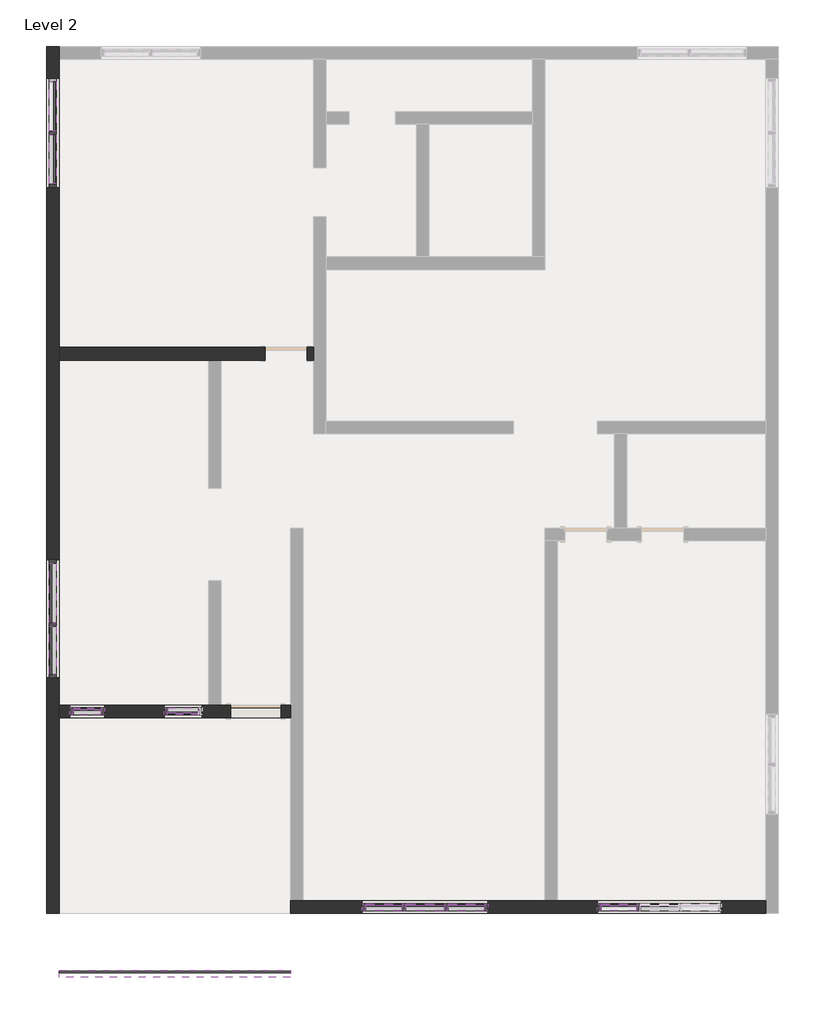
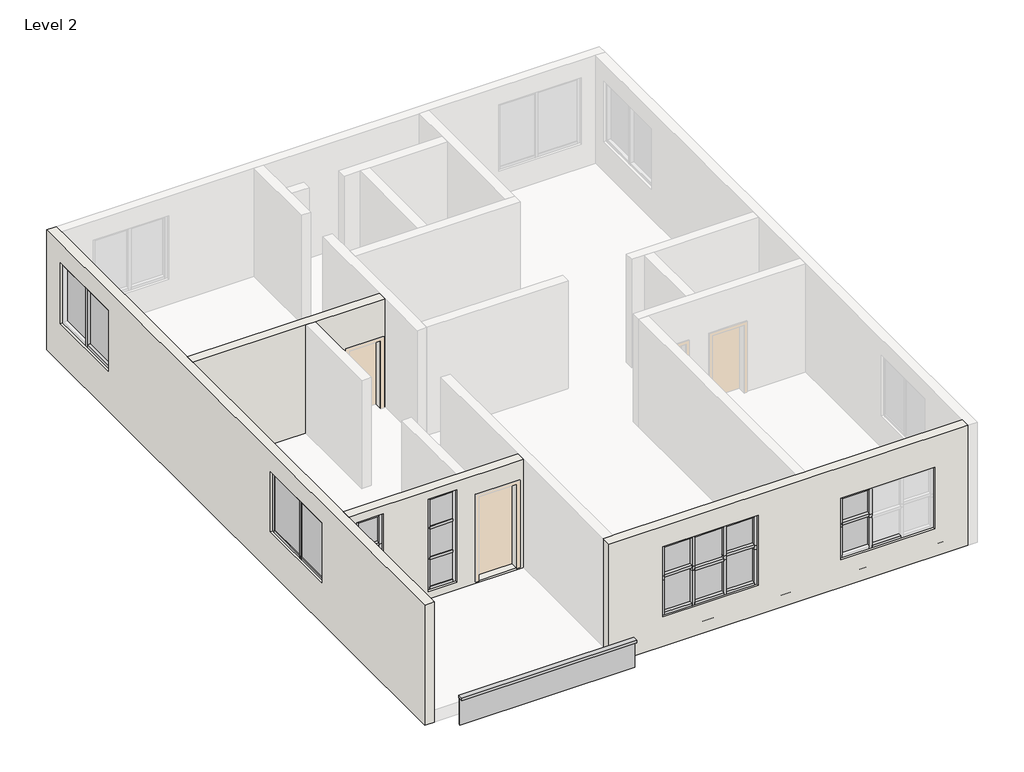
# One storey, part 1 of 2: 60 members, 19 plates, 4 walls.
"""IFC4 building model written with IfcOpenShell, lengths in millimetres."""

from ifc_helpers import new_model, si_unit, origin, place, context, project, spatial, faceted_brep, transform, mapped, element, save
from components import member_00d00b53, member_c7c5a8a0, member_b955a9e9, member_2ee2964b, member_c33c434a, member_3d7cb871, member_f1f71bde, member_024c663a, member_4d6ef9b1, member_a7b21902, member_e5016be8, member_72dfeae6, member_b41a733a, member_7fd687a9, member_90750a43, member_613aa8fe, member_6d419de8, member_bc554fa6, member_50cacee6, member_cfc5edb3, member_fb13da3b, member_24b317d4, member_58fda759, member_d6486fbc, member_c067c3a7, member_db897065, member_a044dc63, member_e51dd2bd, member_dfbe4da1, member_32677b83, member_f4ec938c, member_a37bde81, member_147bebee, system_panel_glazed_4c7522cd, system_panel_glazed_cbd410f7, system_panel_glazed_2af6040d, system_panel_glazed_3f6201ba, system_panel_glazed_11c7b7b5, system_panel_glazed_ea517728, system_panel_glazed_ffb4b76a, system_panel_glazed_52d1a9ac, system_panel_glazed_ee93d072, system_panel_glazed_cb6e72c2, system_panel_glazed_55fd798e, system_panel_glazed_d6f2290d, system_panel_glazed_2cf72723, system_panel_glazed_06e0175a

model = new_model("IFC4")

# Units and contexts
model_context = context("Model", 3, world=origin())
ifc_project = project(units=[si_unit("LENGTHUNIT", "METRE", prefix="MILLI")], contexts=[model_context])

# Site, building, storey
site = spatial("IfcSite", under=ifc_project)
building = spatial("IfcBuilding", under=site)
storey = spatial("IfcBuildingStorey", under=building, Name="Level 2", Elevation=3048.0)

# Members
placement = place(None, origin())
member_shape = member_00d00b53(model_context)
element("IfcMember", 1, ObjectType="Rectangular Mullion : 2.5\" x 5\" rectangular", at=placement, inside=storey, context=model_context, shape_type="MappedRepresentation", body=[
    mapped(member_shape, transform((-8069.267181, -14745.846149, 4532.9555732), x_axis=(1.0, 0.0, 0.0), y_axis=(0.0, -1.0, 0.0), z_axis=(0.0, 0.0, -1.0))),
])
member_2_shape = member_c7c5a8a0(model_context)
element("IfcMember", 2, ObjectType="Rectangular Mullion : 2.5\" x 5\" rectangular", at=placement, inside=storey, context=model_context, shape_type="MappedRepresentation", body=[
    mapped(member_2_shape, transform((-11593.6627168, -14745.846149, 4684.9213312), x_axis=(0.0, 0.0, 1.0), y_axis=(0.0, -1.0, 0.0), z_axis=(1.0, 0.0, 0.0))),
])
member_3_shape = member_b955a9e9(model_context)
element("IfcMember", 3, ObjectType="Rectangular Mullion : 2.5\" x 5\" rectangular", at=placement, inside=storey, context=model_context, shape_type="MappedRepresentation", body=[
    mapped(member_3_shape, transform((-11593.6627168, -14745.846149, 5574.6202549), x_axis=(0.0, 0.0, 1.0), y_axis=(0.0, -1.0, 0.0), z_axis=(1.0, 0.0, 0.0))),
])
element("IfcMember", 4, ObjectType="Rectangular Mullion : 2.5\" x 5\" rectangular", at=placement, inside=storey, context=model_context, shape_type="MappedRepresentation", body=[
    mapped(member_3_shape, transform((-12292.1627168, -14745.846149, 3795.2224075), x_axis=(0.0, 0.0, -1.0), y_axis=(0.0, -1.0, 0.0), z_axis=(-1.0, 0.0, 0.0))),
])
member_4_shape = member_2ee2964b(model_context)
element("IfcMember", 5, ObjectType="Rectangular Mullion : 2.5\" x 5\" rectangular", at=placement, inside=storey, context=model_context, shape_type="MappedRepresentation", body=[
    mapped(member_4_shape, transform((-10863.4127168, -14745.846149, 4786.5213312), x_axis=(0.0, 0.0, 1.0), y_axis=(0.0, -1.0, 0.0), z_axis=(1.0, 0.0, 0.0))),
])
element("IfcMember", 6, ObjectType="Rectangular Mullion : 2.5\" x 5\" rectangular", at=placement, inside=storey, context=model_context, shape_type="MappedRepresentation", body=[
    mapped(member_4_shape, transform((-12355.6627168, -14745.846149, 4786.5213312), x_axis=(0.0, 0.0, 1.0), y_axis=(0.0, -1.0, 0.0), z_axis=(1.0, 0.0, 0.0))),
])
member_5_shape = member_c33c434a(model_context)
element("IfcMember", 7, ObjectType="Rectangular Mullion : 2.5\" x 5\" rectangular", at=placement, inside=storey, context=model_context, shape_type="MappedRepresentation", body=[
    mapped(member_5_shape, transform((-12355.6627168, -14745.846149, 5574.6202549), x_axis=(0.0, 0.0, 1.0), y_axis=(0.0, -1.0, 0.0), z_axis=(1.0, 0.0, 0.0))),
])
element("IfcMember", 8, ObjectType="Rectangular Mullion : 2.5\" x 5\" rectangular", at=placement, inside=storey, context=model_context, shape_type="MappedRepresentation", body=[
    mapped(member_5_shape, transform((-10863.4127168, -14745.846149, 5574.6202549), x_axis=(0.0, 0.0, 1.0), y_axis=(0.0, -1.0, 0.0), z_axis=(1.0, 0.0, 0.0))),
])
element("IfcMember", 9, ObjectType="Rectangular Mullion : 2.5\" x 5\" rectangular", at=placement, inside=storey, context=model_context, shape_type="MappedRepresentation", body=[
    mapped(member_5_shape, transform((-11530.1627168, -14745.846149, 3795.2224075), x_axis=(0.0, 0.0, -1.0), y_axis=(0.0, -1.0, 0.0), z_axis=(-1.0, 0.0, 0.0))),
])
element("IfcMember", 10, ObjectType="Rectangular Mullion : 2.5\" x 5\" rectangular", at=placement, inside=storey, context=model_context, shape_type="MappedRepresentation", body=[
    mapped(member_5_shape, transform((-13022.4127168, -14745.846149, 3795.2224075), x_axis=(0.0, 0.0, -1.0), y_axis=(0.0, -1.0, 0.0), z_axis=(-1.0, 0.0, 0.0))),
])
member_6_shape = member_3d7cb871(model_context)
element("IfcMember", 11, ObjectType="Rectangular Mullion : 2.5\" x 5\" rectangular", at=placement, inside=storey, context=model_context, shape_type="MappedRepresentation", body=[
    mapped(member_6_shape, transform((-8818.7127168, -14745.846149, 4609.1555732), x_axis=(-1.0, 0.0, 0.0), y_axis=(0.0, -1.0, 0.0), z_axis=(0.0, 0.0, 1.0))),
])
member_7_shape = member_f1f71bde(model_context)
element("IfcMember", 12, ObjectType="Rectangular Mullion : 2.5\" x 5\" rectangular", at=placement, inside=storey, context=model_context, shape_type="MappedRepresentation", body=[
    mapped(member_7_shape, transform((-18686.1761094, -756.796149, 4059.4675701), x_axis=(0.0, 0.0, -1.0), y_axis=(-1.0, 0.0, 0.0), z_axis=(0.0, 1.0, 0.0))),
])
element("IfcMember", 13, ObjectType="Rectangular Mullion : 2.5\" x 5\" rectangular", at=placement, inside=storey, context=model_context, shape_type="MappedRepresentation", body=[
    mapped(member_7_shape, transform((-18686.1761094, -693.296149, 5599.1263641), x_axis=(0.0, 0.0, 1.0), y_axis=(-1.0, 0.0, 0.0), z_axis=(0.0, -1.0, 0.0))),
])
element("IfcMember", 14, ObjectType="Rectangular Mullion : 2.5\" x 5\" rectangular", at=placement, inside=storey, context=model_context, shape_type="MappedRepresentation", body=[
    mapped(member_7_shape, transform((-18686.1761094, -1652.146149, 5599.1263641), x_axis=(0.0, 0.0, 1.0), y_axis=(-1.0, 0.0, 0.0), z_axis=(0.0, -1.0, 0.0))),
])
member_8_shape = member_024c663a(model_context)
element("IfcMember", 15, ObjectType="Rectangular Mullion : 2.5\" x 5\" rectangular", at=placement, inside=storey, context=model_context, shape_type="MappedRepresentation", body=[
    mapped(member_8_shape, transform((-18686.1761094, -9659.496149, 5596.1060273), x_axis=(0.0, 0.0, 1.0), y_axis=(1.0, 0.0, 0.0), z_axis=(0.0, 1.0, 0.0))),
])
member_9_shape = member_4d6ef9b1(model_context)
element("IfcMember", 16, ObjectType="Rectangular Mullion : 2.5\" x 5\" rectangular", at=placement, inside=storey, context=model_context, shape_type="MappedRepresentation", body=[
    mapped(member_9_shape, transform((-18686.1761094, -8522.846149, 5596.1060273), x_axis=(0.0, 0.0, 1.0), y_axis=(1.0, 0.0, 0.0), z_axis=(0.0, 1.0, 0.0))),
])
member_10_shape = member_a7b21902(model_context)
element("IfcMember", 17, ObjectType="Rectangular Mullion : 2.5\" x 5\" rectangular", at=placement, inside=storey, context=model_context, shape_type="MappedRepresentation", body=[
    mapped(member_10_shape, transform((-18686.1761094, -9627.746149, 4073.0027042), x_axis=(0.0, 1.0, 0.0), y_axis=(1.0, 0.0, 0.0), z_axis=(0.0, 0.0, -1.0))),
])
element("IfcMember", 18, ObjectType="Rectangular Mullion : 2.5\" x 5\" rectangular", at=placement, inside=storey, context=model_context, shape_type="MappedRepresentation", body=[
    mapped(member_9_shape, transform((-18686.1761094, -9595.996149, 4073.0027042), x_axis=(0.0, 0.0, -1.0), y_axis=(1.0, 0.0, 0.0), z_axis=(0.0, -1.0, 0.0))),
])
element("IfcMember", 19, ObjectType="Rectangular Mullion : 2.5\" x 5\" rectangular", at=placement, inside=storey, context=model_context, shape_type="MappedRepresentation", body=[
    mapped(member_8_shape, transform((-18686.1761094, -10529.446149, 4073.0027042), x_axis=(0.0, 0.0, -1.0), y_axis=(1.0, 0.0, 0.0), z_axis=(0.0, -1.0, 0.0))),
])
member_11_shape = member_e5016be8(model_context)
element("IfcMember", 20, ObjectType="Rectangular Mullion : 2.5\" x 5\" rectangular", at=placement, inside=storey, context=model_context, shape_type="MappedRepresentation", body=[
    mapped(member_11_shape, transform((-18686.1761094, -10592.946149, 5596.1060273), x_axis=(0.0, -1.0, 0.0), y_axis=(1.0, 0.0, 0.0), z_axis=(0.0, 0.0, 1.0))),
])
element("IfcMember", 21, ObjectType="Rectangular Mullion : 2.5\" x 5\" rectangular", at=placement, inside=storey, context=model_context, shape_type="MappedRepresentation", body=[
    mapped(member_11_shape, transform((-18686.1761094, -8459.346149, 4073.0027042), x_axis=(0.0, 1.0, 0.0), y_axis=(1.0, 0.0, 0.0), z_axis=(0.0, 0.0, -1.0))),
])
member_12_shape = member_72dfeae6(model_context)
element("IfcMember", 22, ObjectType="Rectangular Mullion : 2.5\" x 5\" rectangular", at=placement, inside=storey, context=model_context, shape_type="MappedRepresentation", body=[
    mapped(member_12_shape, transform((-18686.1761094, -725.046149, 4059.4675701), x_axis=(0.0, -1.0, 0.0), y_axis=(-1.0, 0.0, 0.0), z_axis=(0.0, 0.0, -1.0))),
])
member_13_shape = member_b41a733a(model_context)
element("IfcMember", 23, ObjectType="Rectangular Mullion : 2.5\" x 5\" rectangular", at=placement, inside=storey, context=model_context, shape_type="MappedRepresentation", body=[
    mapped(member_13_shape, transform((-18686.1761094, -1715.646149, 4059.4675701), x_axis=(0.0, -1.0, 0.0), y_axis=(-1.0, 0.0, 0.0), z_axis=(0.0, 0.0, -1.0))),
])
member_14_shape = member_7fd687a9(model_context)
element("IfcMember", 24, ObjectType="Rectangular Mullion : 2.5\" x 5\" rectangular", at=placement, inside=storey, context=model_context, shape_type="MappedRepresentation", body=[
    mapped(member_14_shape, transform((-17809.8761094, -11202.546149, 5890.7358384), x_axis=(0.0, 0.0, 1.0), y_axis=(0.0, -1.0, 0.0), z_axis=(1.0, 0.0, 0.0))),
])
member_15_shape = member_90750a43(model_context)
element("IfcMember", 25, ObjectType="Rectangular Mullion : 2.5\" x 5\" rectangular", at=placement, inside=storey, context=model_context, shape_type="MappedRepresentation", body=[
    mapped(member_15_shape, transform((-17809.8761094, -11202.546149, 5114.1326107), x_axis=(0.0, 0.0, 1.0), y_axis=(0.0, -1.0, 0.0), z_axis=(1.0, 0.0, 0.0))),
])
element("IfcMember", 26, ObjectType="Rectangular Mullion : 2.5\" x 5\" rectangular", at=placement, inside=storey, context=model_context, shape_type="MappedRepresentation", body=[
    mapped(member_15_shape, transform((-17809.8761094, -11202.546149, 4337.5293829), x_axis=(0.0, 0.0, 1.0), y_axis=(0.0, -1.0, 0.0), z_axis=(1.0, 0.0, 0.0))),
])
member_16_shape = member_613aa8fe(model_context)
element("IfcMember", 27, ObjectType="Rectangular Mullion : 2.5\" x 5\" rectangular", at=placement, inside=storey, context=model_context, shape_type="MappedRepresentation", body=[
    mapped(member_16_shape, transform((-17746.3761094, -11202.546149, 5114.1326107), x_axis=(1.0, 0.0, 0.0), y_axis=(0.0, -1.0, 0.0), z_axis=(0.0, 0.0, -1.0))),
])
element("IfcMember", 28, ObjectType="Rectangular Mullion : 2.5\" x 5\" rectangular", at=placement, inside=storey, context=model_context, shape_type="MappedRepresentation", body=[
    mapped(member_16_shape, transform((-18381.3761094, -11202.546149, 5890.7358384), x_axis=(-1.0, 0.0, 0.0), y_axis=(0.0, -1.0, 0.0), z_axis=(0.0, 0.0, 1.0))),
])
element("IfcMember", 29, ObjectType="Rectangular Mullion : 2.5\" x 5\" rectangular", at=placement, inside=storey, context=model_context, shape_type="MappedRepresentation", body=[
    mapped(member_16_shape, transform((-17746.3761094, -11202.546149, 4337.5293829), x_axis=(1.0, 0.0, 0.0), y_axis=(0.0, -1.0, 0.0), z_axis=(0.0, 0.0, -1.0))),
])
element("IfcMember", 30, ObjectType="Rectangular Mullion : 2.5\" x 5\" rectangular", at=placement, inside=storey, context=model_context, shape_type="MappedRepresentation", body=[
    mapped(member_16_shape, transform((-18381.3761094, -11202.546149, 5114.1326107), x_axis=(-1.0, 0.0, 0.0), y_axis=(0.0, -1.0, 0.0), z_axis=(0.0, 0.0, 1.0))),
])
element("IfcMember", 31, ObjectType="Rectangular Mullion : 2.5\" x 5\" rectangular", at=placement, inside=storey, context=model_context, shape_type="MappedRepresentation", body=[
    mapped(member_14_shape, transform((-18317.8761094, -11202.546149, 3560.9261552), x_axis=(0.0, 0.0, -1.0), y_axis=(0.0, -1.0, 0.0), z_axis=(-1.0, 0.0, 0.0))),
])
element("IfcMember", 32, ObjectType="Rectangular Mullion : 2.5\" x 5\" rectangular", at=placement, inside=storey, context=model_context, shape_type="MappedRepresentation", body=[
    mapped(member_16_shape, transform((-17746.3761094, -11202.546149, 3560.9261552), x_axis=(1.0, 0.0, 0.0), y_axis=(0.0, -1.0, 0.0), z_axis=(0.0, 0.0, -1.0))),
])
element("IfcMember", 33, ObjectType="Rectangular Mullion : 2.5\" x 5\" rectangular", at=placement, inside=storey, context=model_context, shape_type="MappedRepresentation", body=[
    mapped(member_16_shape, transform((-18381.3761094, -11202.546149, 4337.5293829), x_axis=(-1.0, 0.0, 0.0), y_axis=(0.0, -1.0, 0.0), z_axis=(0.0, 0.0, 1.0))),
])
member_17_shape = member_6d419de8(model_context)
element("IfcMember", 34, ObjectType="Rectangular Mullion : 2.5\" x 5\" rectangular", at=placement, inside=storey, context=model_context, shape_type="MappedRepresentation", body=[
    mapped(member_17_shape, transform((-16666.8761094, -11202.546149, 5104.8752687), x_axis=(-1.0, 0.0, 0.0), y_axis=(0.0, 1.0, 0.0), z_axis=(0.0, 0.0, -1.0))),
])
member_18_shape = member_bc554fa6(model_context)
element("IfcMember", 35, ObjectType="Rectangular Mullion : 2.5\" x 5\" rectangular", at=placement, inside=storey, context=model_context, shape_type="MappedRepresentation", body=[
    mapped(member_18_shape, transform((-16603.3761094, -11202.546149, 5104.8752687), x_axis=(0.0, 0.0, 1.0), y_axis=(0.0, 1.0, 0.0), z_axis=(-1.0, 0.0, 0.0))),
])
element("IfcMember", 36, ObjectType="Rectangular Mullion : 2.5\" x 5\" rectangular", at=placement, inside=storey, context=model_context, shape_type="MappedRepresentation", body=[
    mapped(member_18_shape, transform((-16603.3761094, -11202.546149, 4324.942968), x_axis=(0.0, 0.0, 1.0), y_axis=(0.0, 1.0, 0.0), z_axis=(-1.0, 0.0, 0.0))),
])
member_19_shape = member_50cacee6(model_context)
element("IfcMember", 37, ObjectType="Rectangular Mullion : 2.5\" x 5\" rectangular", at=placement, inside=storey, context=model_context, shape_type="MappedRepresentation", body=[
    mapped(member_19_shape, transform((-16603.3761094, -11202.546149, 5884.8075695), x_axis=(0.0, 0.0, 1.0), y_axis=(0.0, 1.0, 0.0), z_axis=(-1.0, 0.0, 0.0))),
])
element("IfcMember", 38, ObjectType="Rectangular Mullion : 2.5\" x 5\" rectangular", at=placement, inside=storey, context=model_context, shape_type="MappedRepresentation", body=[
    mapped(member_17_shape, transform((-16666.8761094, -11202.546149, 4324.942968), x_axis=(-1.0, 0.0, 0.0), y_axis=(0.0, 1.0, 0.0), z_axis=(0.0, 0.0, -1.0))),
])
element("IfcMember", 39, ObjectType="Rectangular Mullion : 2.5\" x 5\" rectangular", at=placement, inside=storey, context=model_context, shape_type="MappedRepresentation", body=[
    mapped(member_19_shape, transform((-16044.5761094, -11202.546149, 3545.0106672), x_axis=(0.0, 0.0, -1.0), y_axis=(0.0, 1.0, 0.0), z_axis=(1.0, 0.0, 0.0))),
])
element("IfcMember", 40, ObjectType="Rectangular Mullion : 2.5\" x 5\" rectangular", at=placement, inside=storey, context=model_context, shape_type="MappedRepresentation", body=[
    mapped(member_17_shape, transform((-16666.8761094, -11202.546149, 3545.0106672), x_axis=(-1.0, 0.0, 0.0), y_axis=(0.0, 1.0, 0.0), z_axis=(0.0, 0.0, -1.0))),
])
member_20_shape = member_cfc5edb3(model_context)
element("IfcMember", 41, ObjectType="Rectangular Mullion : 2.5\" x 5\" rectangular", at=placement, inside=storey, context=model_context, shape_type="MappedRepresentation", body=[
    mapped(member_20_shape, transform((-12323.9127168, -14745.846149, 4684.9213312), x_axis=(1.0, 0.0, 0.0), y_axis=(0.0, -1.0, 0.0), z_axis=(0.0, 0.0, -1.0))),
])
element("IfcMember", 42, ObjectType="Rectangular Mullion : 2.5\" x 5\" rectangular", at=placement, inside=storey, context=model_context, shape_type="MappedRepresentation", body=[
    mapped(member_20_shape, transform((-11561.9127168, -14745.846149, 4684.9213312), x_axis=(1.0, 0.0, 0.0), y_axis=(0.0, -1.0, 0.0), z_axis=(0.0, 0.0, -1.0))),
])
member_21_shape = member_fb13da3b(model_context)
element("IfcMember", 43, ObjectType="Rectangular Mullion : 2.5\" x 5\" rectangular", at=placement, inside=storey, context=model_context, shape_type="MappedRepresentation", body=[
    mapped(member_21_shape, transform((-13085.9127168, -14745.846149, 4786.5213312), x_axis=(-1.0, 0.0, 0.0), y_axis=(0.0, -1.0, 0.0), z_axis=(0.0, 0.0, 1.0))),
])
member_22_shape = member_24b317d4(model_context)
element("IfcMember", 44, ObjectType="Rectangular Mullion : 2.5\" x 5\" rectangular", at=placement, inside=storey, context=model_context, shape_type="MappedRepresentation", body=[
    mapped(member_22_shape, transform((-12323.9127168, -14745.846149, 4786.5213312), x_axis=(1.0, 0.0, 0.0), y_axis=(0.0, -1.0, 0.0), z_axis=(0.0, 0.0, -1.0))),
])
element("IfcMember", 45, ObjectType="Rectangular Mullion : 2.5\" x 5\" rectangular", at=placement, inside=storey, context=model_context, shape_type="MappedRepresentation", body=[
    mapped(member_22_shape, transform((-11561.9127168, -14745.846149, 4786.5213312), x_axis=(1.0, 0.0, 0.0), y_axis=(0.0, -1.0, 0.0), z_axis=(0.0, 0.0, -1.0))),
])
member_23_shape = member_58fda759(model_context)
element("IfcMember", 46, ObjectType="Rectangular Mullion : 2.5\" x 5\" rectangular", at=placement, inside=storey, context=model_context, shape_type="MappedRepresentation", body=[
    mapped(member_23_shape, transform((-13085.9127168, -14745.846149, 5574.6202549), x_axis=(-1.0, 0.0, 0.0), y_axis=(0.0, -1.0, 0.0), z_axis=(0.0, 0.0, 1.0))),
])
element("IfcMember", 47, ObjectType="Rectangular Mullion : 2.5\" x 5\" rectangular", at=placement, inside=storey, context=model_context, shape_type="MappedRepresentation", body=[
    mapped(member_23_shape, transform((-10799.9127168, -14745.846149, 4786.5213312), x_axis=(1.0, 0.0, 0.0), y_axis=(0.0, -1.0, 0.0), z_axis=(0.0, 0.0, -1.0))),
])
element("IfcMember", 48, ObjectType="Rectangular Mullion : 2.5\" x 5\" rectangular", at=placement, inside=storey, context=model_context, shape_type="MappedRepresentation", body=[
    mapped(member_21_shape, transform((-10799.9127168, -14745.846149, 4684.9213312), x_axis=(1.0, 0.0, 0.0), y_axis=(0.0, -1.0, 0.0), z_axis=(0.0, 0.0, -1.0))),
])
member_24_shape = member_d6486fbc(model_context)
element("IfcMember", 49, ObjectType="Rectangular Mullion : 2.5\" x 5\" rectangular", at=placement, inside=storey, context=model_context, shape_type="MappedRepresentation", body=[
    mapped(member_24_shape, transform((-12323.9127168, -14745.846149, 3795.2224075), x_axis=(1.0, 0.0, 0.0), y_axis=(0.0, -1.0, 0.0), z_axis=(0.0, 0.0, -1.0))),
])
element("IfcMember", 50, ObjectType="Rectangular Mullion : 2.5\" x 5\" rectangular", at=placement, inside=storey, context=model_context, shape_type="MappedRepresentation", body=[
    mapped(member_24_shape, transform((-11561.9127168, -14745.846149, 3795.2224075), x_axis=(1.0, 0.0, 0.0), y_axis=(0.0, -1.0, 0.0), z_axis=(0.0, 0.0, -1.0))),
])
member_25_shape = member_c067c3a7(model_context)
element("IfcMember", 51, ObjectType="Rectangular Mullion : 2.5\" x 5\" rectangular", at=placement, inside=storey, context=model_context, shape_type="MappedRepresentation", body=[
    mapped(member_25_shape, transform((-13085.9127168, -14745.846149, 4684.9213312), x_axis=(-1.0, 0.0, 0.0), y_axis=(0.0, -1.0, 0.0), z_axis=(0.0, 0.0, 1.0))),
])
element("IfcMember", 52, ObjectType="Rectangular Mullion : 2.5\" x 5\" rectangular", at=placement, inside=storey, context=model_context, shape_type="MappedRepresentation", body=[
    mapped(member_25_shape, transform((-10799.9127168, -14745.846149, 3795.2224075), x_axis=(1.0, 0.0, 0.0), y_axis=(0.0, -1.0, 0.0), z_axis=(0.0, 0.0, -1.0))),
])
member_26_shape = member_db897065(model_context)
element("IfcMember", 53, ObjectType="Rectangular Mullion : 2.5\" x 5\" rectangular", at=placement, inside=storey, context=model_context, shape_type="MappedRepresentation", body=[
    mapped(member_26_shape, transform((-8069.267181, -14745.846149, 4609.1555732), x_axis=(1.0, 0.0, 0.0), y_axis=(0.0, -1.0, 0.0), z_axis=(0.0, 0.0, -1.0))),
])
member_27_shape = member_a044dc63(model_context)
element("IfcMember", 54, ObjectType="Rectangular Mullion : 2.5\" x 5\" rectangular", at=placement, inside=storey, context=model_context, shape_type="MappedRepresentation", body=[
    mapped(member_27_shape, transform((-8101.017181, -14745.846149, 5311.3816242), x_axis=(0.0, 0.0, 1.0), y_axis=(0.0, -1.0, 0.0), z_axis=(1.0, 0.0, 0.0))),
])
member_28_shape = member_e51dd2bd(model_context)
element("IfcMember", 55, ObjectType="Rectangular Mullion : 2.5\" x 5\" rectangular", at=placement, inside=storey, context=model_context, shape_type="MappedRepresentation", body=[
    mapped(member_28_shape, transform((-8101.017181, -14745.846149, 4609.1555732), x_axis=(0.0, 0.0, 1.0), y_axis=(0.0, -1.0, 0.0), z_axis=(1.0, 0.0, 0.0))),
])
member_29_shape = member_dfbe4da1(model_context)
element("IfcMember", 56, ObjectType="Rectangular Mullion : 2.5\" x 5\" rectangular", at=placement, inside=storey, context=model_context, shape_type="MappedRepresentation", body=[
    mapped(member_29_shape, transform((-8818.7127168, -14745.846149, 5311.3816242), x_axis=(-1.0, 0.0, 0.0), y_axis=(0.0, -1.0, 0.0), z_axis=(0.0, 0.0, 1.0))),
])
member_30_shape = member_32677b83(model_context)
element("IfcMember", 57, ObjectType="Rectangular Mullion : 2.5\" x 5\" rectangular", at=placement, inside=storey, context=model_context, shape_type="MappedRepresentation", body=[
    mapped(member_30_shape, transform((-8069.267181, -14745.846149, 3754.5295223), x_axis=(1.0, 0.0, 0.0), y_axis=(0.0, -1.0, 0.0), z_axis=(0.0, 0.0, -1.0))),
])
member_31_shape = member_f4ec938c(model_context)
element("IfcMember", 58, ObjectType="Rectangular Mullion : 2.5\" x 5\" rectangular", at=placement, inside=storey, context=model_context, shape_type="MappedRepresentation", body=[
    mapped(member_31_shape, transform((-8037.517181, -14745.846149, 3754.5295223), x_axis=(0.0, 0.0, -1.0), y_axis=(0.0, -1.0, 0.0), z_axis=(-1.0, 0.0, 0.0))),
])
member_32_shape = member_a37bde81(model_context)
element("IfcMember", 59, ObjectType="Rectangular Mullion : 2.5\" x 5\" rectangular", at=placement, inside=storey, context=model_context, shape_type="MappedRepresentation", body=[
    mapped(member_32_shape, transform((-8818.7127168, -14745.846149, 4532.9555732), x_axis=(-1.0, 0.0, 0.0), y_axis=(0.0, -1.0, 0.0), z_axis=(0.0, 0.0, 1.0))),
])
member_33_shape = member_147bebee(model_context)
element("IfcMember", 60, ObjectType="Rectangular Mullion : 2.5\" x 5\" rectangular", at=placement, inside=storey, context=model_context, shape_type="MappedRepresentation", body=[
    mapped(member_33_shape, transform((-14380.8761094, -15957.1913837, 4356.692968), x_axis=(0.0, 0.0, 1.0), y_axis=(0.0, -1.0, 0.0), z_axis=(1.0, 0.0, 0.0))),
])

# Plates
system_panel_glazed_shape = system_panel_glazed_4c7522cd(model_context)
element("IfcPlate", 61, ObjectType="System Panel : Glazed", at=placement, inside=storey, context=model_context, shape_type="MappedRepresentation", body=[
    mapped(system_panel_glazed_shape, transform((-18686.1761094, -10094.471149, 4136.5027042), x_axis=(0.0, 1.0, 0.0), y_axis=(-1.0, 0.0, 0.0), z_axis=(0.0, 0.0, 1.0))),
])
system_panel_glazed_2_shape = system_panel_glazed_cbd410f7(model_context)
element("IfcPlate", 62, ObjectType="System Panel : Glazed", at=placement, inside=storey, context=model_context, shape_type="MappedRepresentation", body=[
    mapped(system_panel_glazed_2_shape, transform((-18686.1761094, -9059.421149, 4136.5027042), x_axis=(0.0, 1.0, 0.0), y_axis=(-1.0, 0.0, 0.0), z_axis=(0.0, 0.0, 1.0))),
])
system_panel_glazed_3_shape = system_panel_glazed_2af6040d(model_context)
element("IfcPlate", 63, ObjectType="System Panel : Glazed", at=placement, inside=storey, context=model_context, shape_type="MappedRepresentation", body=[
    mapped(system_panel_glazed_3_shape, transform((-18686.1761094, -245.621149, 4122.9675701), x_axis=(0.0, -1.0, 0.0), y_axis=(1.0, 0.0, 0.0), z_axis=(0.0, 0.0, 1.0))),
])
element("IfcPlate", 64, ObjectType="System Panel : Glazed", at=placement, inside=storey, context=model_context, shape_type="MappedRepresentation", body=[
    mapped(system_panel_glazed_3_shape, transform((-18686.1761094, -1204.471149, 4122.9675701), x_axis=(0.0, -1.0, 0.0), y_axis=(1.0, 0.0, 0.0), z_axis=(0.0, 0.0, 1.0))),
])
system_panel_glazed_4_shape = system_panel_glazed_3f6201ba(model_context)
element("IfcPlate", 65, ObjectType="System Panel : Glazed", at=placement, inside=storey, context=model_context, shape_type="MappedRepresentation", body=[
    mapped(system_panel_glazed_4_shape, transform((-18063.8761094, -11202.546149, 3624.4261552), x_axis=(1.0, 0.0, 0.0), y_axis=(0.0, 1.0, 0.0), z_axis=(0.0, 0.0, 1.0))),
])
element("IfcPlate", 66, ObjectType="System Panel : Glazed", at=placement, inside=storey, context=model_context, shape_type="MappedRepresentation", body=[
    mapped(system_panel_glazed_4_shape, transform((-18063.8761094, -11202.546149, 5145.8826107), x_axis=(1.0, 0.0, 0.0), y_axis=(0.0, 1.0, 0.0), z_axis=(0.0, 0.0, 1.0))),
])
system_panel_glazed_5_shape = system_panel_glazed_11c7b7b5(model_context)
element("IfcPlate", 67, ObjectType="System Panel : Glazed", at=placement, inside=storey, context=model_context, shape_type="MappedRepresentation", body=[
    mapped(system_panel_glazed_5_shape, transform((-18063.8761094, -11202.546149, 4369.2793829), x_axis=(1.0, 0.0, 0.0), y_axis=(0.0, 1.0, 0.0), z_axis=(0.0, 0.0, 1.0))),
])
system_panel_glazed_6_shape = system_panel_glazed_ea517728(model_context)
element("IfcPlate", 68, ObjectType="System Panel : Glazed", at=placement, inside=storey, context=model_context, shape_type="MappedRepresentation", body=[
    mapped(system_panel_glazed_6_shape, transform((-16323.9761094, -11202.546149, 3608.5106672), x_axis=(-1.0, 0.0, 0.0), y_axis=(0.0, -1.0, 0.0), z_axis=(0.0, 0.0, 1.0))),
])
element("IfcPlate", 69, ObjectType="System Panel : Glazed", at=placement, inside=storey, context=model_context, shape_type="MappedRepresentation", body=[
    mapped(system_panel_glazed_6_shape, transform((-16323.9761094, -11202.546149, 5136.6252687), x_axis=(-1.0, 0.0, 0.0), y_axis=(0.0, -1.0, 0.0), z_axis=(0.0, 0.0, 1.0))),
])
system_panel_glazed_7_shape = system_panel_glazed_ffb4b76a(model_context)
element("IfcPlate", 70, ObjectType="System Panel : Glazed", at=placement, inside=storey, context=model_context, shape_type="MappedRepresentation", body=[
    mapped(system_panel_glazed_7_shape, transform((-16323.9761094, -11202.546149, 4356.692968), x_axis=(-1.0, 0.0, 0.0), y_axis=(0.0, -1.0, 0.0), z_axis=(0.0, 0.0, 1.0))),
])
system_panel_glazed_8_shape = system_panel_glazed_52d1a9ac(model_context)
element("IfcPlate", 71, ObjectType="System Panel : Glazed", at=placement, inside=storey, context=model_context, shape_type="MappedRepresentation", body=[
    mapped(system_panel_glazed_8_shape, transform((-12689.0377168, -14745.846149, 4818.2713312), x_axis=(1.0, 0.0, 0.0), y_axis=(0.0, 1.0, 0.0), z_axis=(0.0, 0.0, 1.0))),
])
element("IfcPlate", 72, ObjectType="System Panel : Glazed", at=placement, inside=storey, context=model_context, shape_type="MappedRepresentation", body=[
    mapped(system_panel_glazed_8_shape, transform((-11196.7877168, -14745.846149, 4818.2713312), x_axis=(1.0, 0.0, 0.0), y_axis=(0.0, 1.0, 0.0), z_axis=(0.0, 0.0, 1.0))),
])
system_panel_glazed_9_shape = system_panel_glazed_ee93d072(model_context)
element("IfcPlate", 73, ObjectType="System Panel : Glazed", at=placement, inside=storey, context=model_context, shape_type="MappedRepresentation", body=[
    mapped(system_panel_glazed_9_shape, transform((-11942.9127168, -14745.846149, 4716.6713312), x_axis=(1.0, 0.0, 0.0), y_axis=(0.0, 1.0, 0.0), z_axis=(0.0, 0.0, 1.0))),
])
system_panel_glazed_10_shape = system_panel_glazed_cb6e72c2(model_context)
element("IfcPlate", 74, ObjectType="System Panel : Glazed", at=placement, inside=storey, context=model_context, shape_type="MappedRepresentation", body=[
    mapped(system_panel_glazed_10_shape, transform((-12689.0377168, -14745.846149, 3858.7224075), x_axis=(1.0, 0.0, 0.0), y_axis=(0.0, 1.0, 0.0), z_axis=(0.0, 0.0, 1.0))),
])
element("IfcPlate", 75, ObjectType="System Panel : Glazed", at=placement, inside=storey, context=model_context, shape_type="MappedRepresentation", body=[
    mapped(system_panel_glazed_10_shape, transform((-11196.7877168, -14745.846149, 3858.7224075), x_axis=(1.0, 0.0, 0.0), y_axis=(0.0, 1.0, 0.0), z_axis=(0.0, 0.0, 1.0))),
])
system_panel_glazed_11_shape = system_panel_glazed_55fd798e(model_context)
element("IfcPlate", 76, ObjectType="System Panel : Glazed", at=placement, inside=storey, context=model_context, shape_type="MappedRepresentation", body=[
    mapped(system_panel_glazed_11_shape, transform((-11942.9127168, -14745.846149, 3858.7224075), x_axis=(1.0, 0.0, 0.0), y_axis=(0.0, 1.0, 0.0), z_axis=(0.0, 0.0, 1.0))),
])
system_panel_glazed_12_shape = system_panel_glazed_d6f2290d(model_context)
element("IfcPlate", 77, ObjectType="System Panel : Glazed", at=placement, inside=storey, context=model_context, shape_type="MappedRepresentation", body=[
    mapped(system_panel_glazed_12_shape, transform((-8428.1149489, -14745.846149, 4640.9055732), x_axis=(1.0, 0.0, 0.0), y_axis=(0.0, 1.0, 0.0), z_axis=(0.0, 0.0, 1.0))),
])
system_panel_glazed_13_shape = system_panel_glazed_2cf72723(model_context)
element("IfcPlate", 78, ObjectType="System Panel : Glazed", at=placement, inside=storey, context=model_context, shape_type="MappedRepresentation", body=[
    mapped(system_panel_glazed_13_shape, transform((-8428.1149489, -14745.846149, 3818.0295223), x_axis=(1.0, 0.0, 0.0), y_axis=(0.0, 1.0, 0.0), z_axis=(0.0, 0.0, 1.0))),
])
system_panel_glazed_14_shape = system_panel_glazed_06e0175a(model_context)
element("IfcPlate", 79, ObjectType="System Panel : Glazed", at=placement, inside=storey, context=model_context, shape_type="MappedRepresentation", body=[
    mapped(system_panel_glazed_14_shape, transform((-16476.3761094, -15957.1913837, 3630.9088336), x_axis=(1.0, 0.0, 0.0), y_axis=(0.0, 1.0, 0.0), z_axis=(0.0, 0.0, 1.0))),
])

# Walls
element("IfcWall", 80, ObjectType="9\"", at=placement, inside=storey, context=model_context, shape_type="Brep", body=[
    faceted_brep([(-18571.8761094, -14860.146149, 3048.0), (-18571.8761094, -11316.846149, 3048.0), (-18571.8761094, -11088.246149, 3048.0), (-18571.8761094, -4839.846149, 3048.0), (-18571.8761094, -4611.246149, 3048.0), (-18571.8761094, 608.453851, 3048.0), (-18571.8761094, 837.053851, 3048.0), (-18571.8761094, 837.053851, 6096.0), (-18571.8761094, 608.453851, 6096.0), (-18571.8761094, -4611.246149, 6096.0), (-18571.8761094, -4839.846149, 6096.0), (-18571.8761094, -11088.246149, 6096.0), (-18571.8761094, -11316.846149, 6096.0), (-18571.8761094, -14860.146149, 6096.0), (-18571.8761094, 265.553851, 5599.1263641), (-18571.8761094, 265.553851, 4059.4675701), (-18571.8761094, -1715.646149, 4059.4675701), (-18571.8761094, -1715.646149, 5599.1263641), (-18571.8761094, -10592.946149, 4073.0027042), (-18571.8761094, -10592.946149, 5596.1060273), (-18571.8761094, -8459.346149, 5596.1060273), (-18571.8761094, -8459.346149, 4073.0027042), (-18800.4761094, 837.053851, 3048.0), (-18800.4761094, -14860.146149, 3048.0), (-18800.4761094, -14860.146149, 6096.0), (-18800.4761094, 837.053851, 6096.0), (-18800.4761094, 265.553851, 4059.4675701), (-18800.4761094, 265.553851, 5599.1263641), (-18800.4761094, -1715.646149, 5599.1263641), (-18800.4761094, -1715.646149, 4059.4675701), (-18800.4761094, -10592.946149, 5596.1060273), (-18800.4761094, -10592.946149, 4073.0027042), (-18800.4761094, -8459.346149, 4073.0027042), (-18800.4761094, -8459.346149, 5596.1060273)], [[[0, 1, 2, 3, 4, 5, 6, 7, 8, 9, 10, 11, 12, 13], [14, 15, 16, 17], [18, 19, 20, 21]], [[22, 23, 24, 25], [26, 27, 28, 29], [30, 31, 32, 33]], [[6, 5, 4, 3, 2, 1, 0, 23, 22]], [[13, 12, 11, 10, 9, 8, 7, 25, 24]], [[0, 13, 24, 23]], [[7, 6, 22, 25]], [[26, 15, 14, 27]], [[27, 14, 17, 28]], [[28, 17, 16, 29]], [[15, 26, 29, 16]], [[30, 19, 18, 31]], [[19, 30, 33, 20]], [[20, 33, 32, 21]], [[31, 18, 21, 32]]]),
])
element("IfcWall", 81, ObjectType="9\"", at=placement, inside=storey, context=model_context, shape_type="Brep", body=[
    faceted_brep([(-5770.2761094, -14631.546149, 3048.0), (-9542.1761094, -14631.546149, 3048.0), (-9770.7761094, -14631.546149, 3048.0), (-14152.2761094, -14631.546149, 3048.0), (-14380.8761094, -14631.546149, 3048.0), (-14380.8761094, -14631.546149, 6096.0), (-14152.2761094, -14631.546149, 6096.0), (-9770.7761094, -14631.546149, 6096.0), (-9542.1761094, -14631.546149, 6096.0), (-5770.2761094, -14631.546149, 6096.0), (-13085.9127168, -14631.546149, 5574.6202549), (-13085.9127168, -14631.546149, 3795.2224075), (-10799.9127168, -14631.546149, 3795.2224075), (-10799.9127168, -14631.546149, 5574.6202549), (-8818.7127168, -14631.546149, 5311.3816242), (-8818.7127168, -14631.546149, 3754.5295223), (-6570.3761094, -14631.546149, 3754.5295223), (-6570.3761094, -14631.546149, 5311.3816242), (-14380.8761094, -14860.146149, 3048.0), (-5770.2761094, -14860.146149, 3048.0), (-5770.2761094, -14860.146149, 6096.0), (-14380.8761094, -14860.146149, 6096.0), (-13085.9127168, -14860.146149, 3795.2224075), (-13085.9127168, -14860.146149, 5574.6202549), (-10799.9127168, -14860.146149, 5574.6202549), (-10799.9127168, -14860.146149, 3795.2224075), (-8818.7127168, -14860.146149, 3754.5295223), (-8818.7127168, -14860.146149, 5311.3816242), (-6570.3761094, -14860.146149, 5311.3816242), (-6570.3761094, -14860.146149, 3754.5295223)], [[[0, 1, 2, 3, 4, 5, 6, 7, 8, 9], [10, 11, 12, 13], [14, 15, 16, 17]], [[18, 19, 20, 21], [22, 23, 24, 25], [26, 27, 28, 29]], [[4, 3, 2, 1, 0, 19, 18]], [[9, 8, 7, 6, 5, 21, 20]], [[0, 9, 20, 19]], [[5, 4, 18, 21]], [[10, 23, 22, 11]], [[23, 10, 13, 24]], [[24, 13, 12, 25]], [[11, 22, 25, 12]], [[26, 15, 14, 27]], [[27, 14, 17, 28]], [[28, 17, 16, 29]], [[15, 26, 29, 16]]]),
])
element("IfcWall", 82, ObjectType="9\"", at=placement, inside=storey, context=model_context, shape_type="Brep", body=[
    faceted_brep([(-14380.8761094, -11088.246149, 3048.0), (-15638.1761094, -11088.246149, 3048.0), (-15866.7761094, -11088.246149, 3048.0), (-18571.8761094, -11088.246149, 3048.0), (-18571.8761094, -11088.246149, 6096.0), (-15866.7761094, -11088.246149, 6096.0), (-15638.1761094, -11088.246149, 6096.0), (-14380.8761094, -11088.246149, 6096.0), (-15466.7261094, -11088.246149, 3403.6), (-14552.3261094, -11088.246149, 3403.6), (-14552.3261094, -11088.246149, 5537.2), (-15466.7261094, -11088.246149, 5537.2), (-15981.0761094, -11088.246149, 3545.0106672), (-15981.0761094, -11088.246149, 5884.8075695), (-16666.8761094, -11088.246149, 5884.8075695), (-16666.8761094, -11088.246149, 3545.0106672), (-18381.3761094, -11088.246149, 5890.7358384), (-18381.3761094, -11088.246149, 3560.9261552), (-17746.3761094, -11088.246149, 3560.9261552), (-17746.3761094, -11088.246149, 5890.7358384), (-18571.8761094, -11316.846149, 3048.0), (-14380.8761094, -11316.846149, 3048.0), (-14380.8761094, -11316.846149, 6096.0), (-18571.8761094, -11316.846149, 6096.0), (-14552.3261094, -11316.846149, 3403.6), (-15466.7261094, -11316.846149, 3403.6), (-15466.7261094, -11316.846149, 5537.2), (-14552.3261094, -11316.846149, 5537.2), (-15981.0761094, -11316.846149, 5884.8075695), (-15981.0761094, -11316.846149, 3545.0106672), (-16666.8761094, -11316.846149, 3545.0106672), (-16666.8761094, -11316.846149, 5884.8075695), (-18381.3761094, -11316.846149, 3560.9261552), (-18381.3761094, -11316.846149, 5890.7358384), (-17746.3761094, -11316.846149, 5890.7358384), (-17746.3761094, -11316.846149, 3560.9261552)], [[[0, 1, 2, 3, 4, 5, 6, 7], [8, 9, 10, 11], [12, 13, 14, 15], [16, 17, 18, 19]], [[20, 21, 22, 23], [24, 25, 26, 27], [28, 29, 30, 31], [32, 33, 34, 35]], [[3, 2, 1, 0, 21, 20]], [[7, 6, 5, 4, 23, 22]], [[0, 7, 22, 21]], [[4, 3, 20, 23]], [[9, 8, 25, 24]], [[10, 9, 24, 27]], [[11, 10, 27, 26]], [[8, 11, 26, 25]], [[12, 29, 28, 13]], [[13, 28, 31, 14]], [[14, 31, 30, 15]], [[29, 12, 15, 30]], [[32, 17, 16, 33]], [[33, 16, 19, 34]], [[18, 35, 34, 19]], [[17, 32, 35, 18]]]),
])
element("IfcWall", 83, ObjectType="9\"", at=placement, inside=storey, context=model_context, shape_type="Brep", body=[
    faceted_brep([(-14076.5127168, -4839.846149, 5080.0), (-14076.5127168, -4839.846149, 3048.0), (-13962.2127168, -4839.846149, 3048.0), (-13962.2127168, -4839.846149, 6096.0), (-15638.1761094, -4839.846149, 6096.0), (-15866.7761094, -4839.846149, 6096.0), (-18571.8761094, -4839.846149, 6096.0), (-18571.8761094, -4839.846149, 3048.0), (-15866.7761094, -4839.846149, 3048.0), (-15638.1761094, -4839.846149, 3048.0), (-14838.5127168, -4839.846149, 3048.0), (-14838.5127168, -4839.846149, 5080.0), (-13962.2127168, -4611.246149, 3048.0), (-14076.5127168, -4611.246149, 3048.0), (-14076.5127168, -4611.246149, 5080.0), (-14838.5127168, -4611.246149, 5080.0), (-14838.5127168, -4611.246149, 3048.0), (-18571.8761094, -4611.246149, 3048.0), (-18571.8761094, -4611.246149, 6096.0), (-13962.2127168, -4611.246149, 6096.0)], [[[0, 1, 2, 3, 4, 5, 6, 7, 8, 9, 10, 11]], [[12, 13, 14, 15, 16, 17, 18, 19]], [[2, 1, 13, 12]], [[10, 9, 8, 7, 17, 16]], [[6, 5, 4, 3, 19, 18]], [[7, 6, 18, 17]], [[3, 2, 12, 19]], [[14, 13, 1, 0]], [[15, 14, 0, 11]], [[16, 15, 11, 10]]]),
])

save(model, "model.ifc")

# Revit data of these elements
# Type "Rectangular Mullion : 2.5\" x 5\" rectangular"
#   built-in parameter 1007304 = 0.416667 (stored number, unit not read)
#   built-in parameter 1007301 = 0.104167 (stored number, unit not read)
#   built-in parameter 1007300 = 0.104167 (stored number, unit not read)
# Type "System Panel : Glazed"
#   Construction Type Id = "GSP4R"
#   Analytic Construction = "1/8 in Pilkington single glazing"
#   Visual Light Transmittance = 0.9
#   Solar Heat Gain Coefficient = 0.86
#   Heat Transfer Coefficient (U) = 1.18115 BTU/(h·ft²·°F)
#   Define Thermal Properties by = 1
# Type "9\""
#   Assembly Code = "B2010"
#   Layers, outside or top first: 0' - 9" no material (function 1)
# Elements 1, 2, 3, 4, 5, 6, 7, 8, 9, 10, 11, 12, 13, 14, 15, 16, 17, 18, 19, 20, 21, 22, 23, 24, 25, 26, 27, 28, 29, 30, 31, 32, 33, 34, 35, 36, 37, 38, 39, 40, 41, 42, 43, 44, 45, 46, 47, 48, 49, 50, 51, 52, 53, 54, 55, 56, 57, 58, 59, 60 (IfcMember, "Rectangular Mullion : 2.5\" x 5\" rectangular")
#   Phase Created = New Construction
#   Materials on its faces: "Aluminum"
# Elements 61, 62, 63, 64, 65, 66, 67, 68, 69, 70, 71, 72, 73, 74, 75, 76, 77, 78, 79 (IfcPlate, "System Panel : Glazed")
#   Phase Created = New Construction
#   Materials on its faces: "Glass"
# Elements 80, 81, 82, 83 (IfcWall, "9\"")
#   Top Offset = 0' - 0"
#   Base Offset = 0' - 0"
#   Unconnected Height = 10' - 0"
#   wall height = 10' - 0"
#   Phase Created = New Construction
#   Base Constraint = Level 2
#   Materials on its faces: "Default Wall"
# Materials
#   "Aluminum": class "Metal", colour RGB 247 247 247, transparency 0, Description = "Aluminum 6061", Cost = 0
#   "Glass": class "Glass", colour RGB 0 128 192, transparency 0.75, Description = "Soda Lime Glass", Cost = 0
#   "Default Wall": colour RGB 128 128 128, transparency 0, Cost = 0
